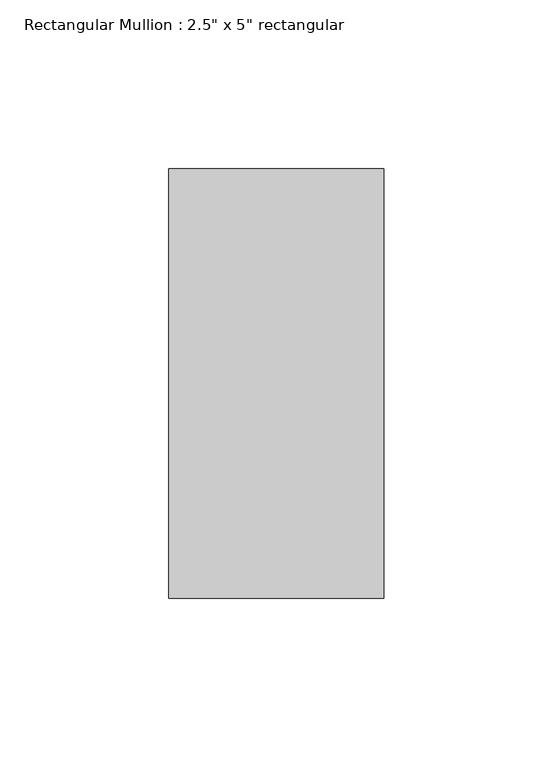
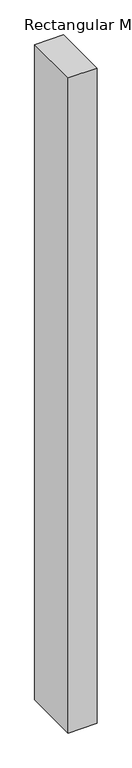
"""IFC4 building model written with IfcOpenShell, lengths in millimetres: member geometry."""

from ifc_helpers import new_model, si_unit, frame, origin, place, context, project, spatial, polyline, outline, extrude, source, transform, mapped, element, save


def member_32e692cc(model_context):
    return source(origin(), model_context, "Body", "SweptSolid", [
        extrude(outline(polyline([(31.75, 63.5), (31.75, -63.5), (-31.75, -63.5), (-31.75, 63.5), (31.75, 63.5)])), frame((0.0, 0.0, -1516.4056705), z_axis=(0.0, 0.0, 1.0), x_axis=(1.0, 0.0, 0.0)), (0.0, 0.0, 1.0), 1516.4056705),
    ])


if __name__ == "__main__":
    model = new_model("IFC4")
    model_context = context("Model", 3, world=origin())
    ifc_project = project(units=[si_unit("LENGTHUNIT", "METRE", prefix="MILLI")], contexts=[model_context])
    site = spatial("IfcSite", under=ifc_project)
    building = spatial("IfcBuilding", under=site)
    placement = place(None, origin())
    member_shape = member_32e692cc(model_context)
    element("IfcMember", 1, ObjectType="Rectangular Mullion : 2.5\" x 5\" rectangular", at=placement, inside=building, context=model_context, shape_type="MappedRepresentation", body=[
        mapped(member_shape, transform((0.0, 0.0, 0.0), x_axis=(1.0, 0.0, 0.0), y_axis=(0.0, 1.0, 0.0), z_axis=(0.0, 0.0, 1.0))),
    ])
    save(model, "model.ifc")

# Revit data of these elements
# Type "Rectangular Mullion : 2.5\" x 5\" rectangular"
#   built-in parameter 1007304 = 0.416667 (stored number, unit not read)
#   built-in parameter 1007301 = 0.104167 (stored number, unit not read)
#   built-in parameter 1007300 = 0.104167 (stored number, unit not read)
# Element 1 (IfcMember, "Rectangular Mullion : 2.5\" x 5\" rectangular")
#   Materials on its faces: "Aluminum"
# Materials
#   "Aluminum": class "Metal", colour RGB 247 247 247, transparency 0, Description = "Aluminum 6061", Cost = 0
